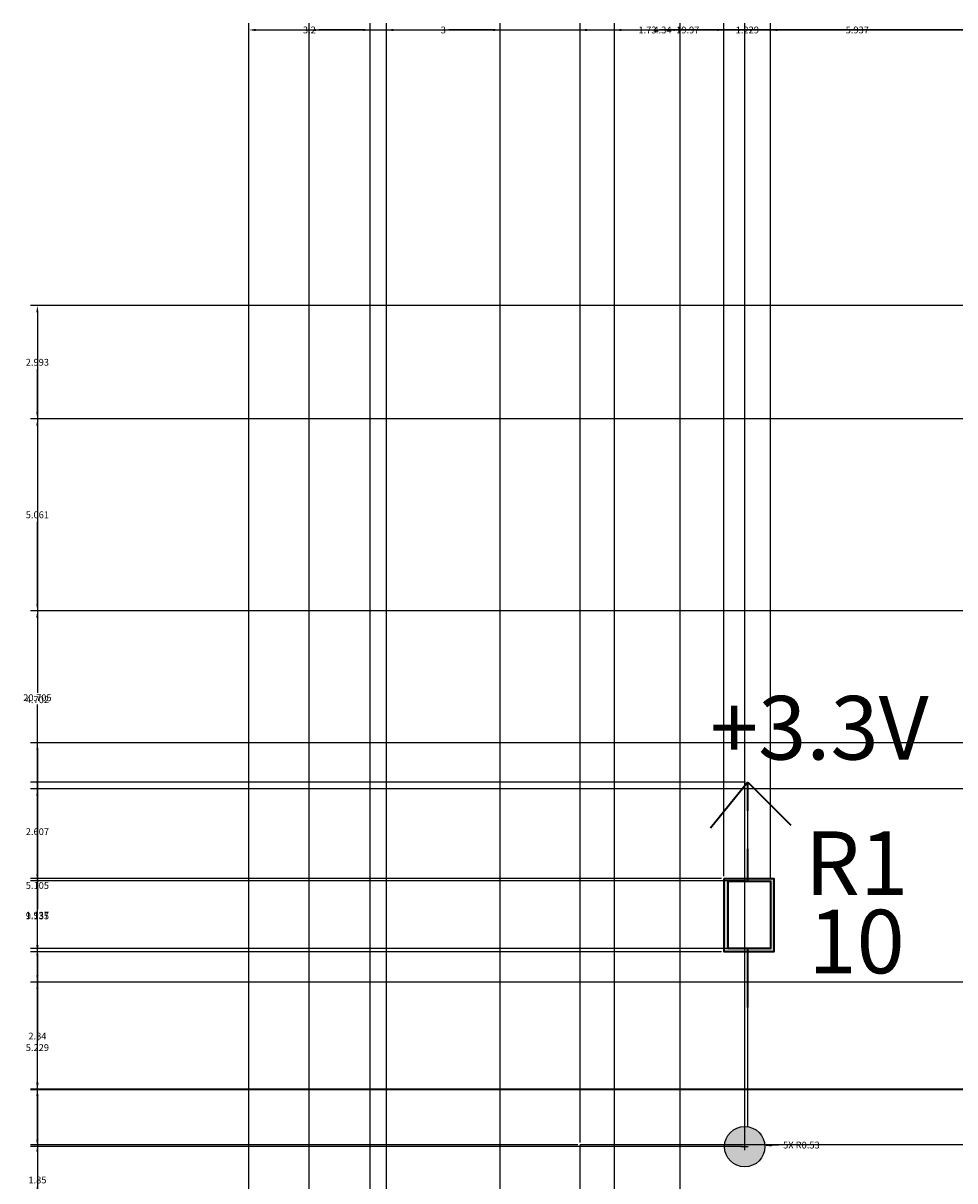
# Model space of a CAD drawing. Units: inches. Extents: x 23 to 132, y 5 to 105.
# Tile 3 of 14: x 23 to 47, y 75 to 105. Entities that reach past the tile are written whole.
import ezdxf

# ---------------------------------------------------------------- set-up
doc = ezdxf.new("R2010")
doc.units = ezdxf.units.IN
doc.header["$MEASUREMENT"] = 0
for name, color, linetype, lineweight in [('A-ANNO-DIMS', 2, 'Continuous', 18), ('E-ANNO-IDEN', 4, 'Continuous', 18), ('E-SYMB', 1, 'Continuous', 35), ('E-SYMB-PATT', 1, 'Continuous', 18), ('E-WIRE', 3, 'Continuous', 25), ('E-WIRE-PATT', 3, 'Continuous', 18)]:
    doc.layers.add(name, color=color, linetype=linetype, lineweight=lineweight)
doc.styles.get("Standard").update_dxf_attribs({"font": 'arial.ttf'})
doc.dimstyles.get("Standard").update_dxf_attribs({"dimtxt": 0.18, "dimasz": 0.18, "dimexe": 0.18, "dimexo": 0.0625, "dimgap": 0.09, "dimtad": 0, "dimtih": 1, "dimtoh": 1, "dimdec": 4, "dimzin": 0, "dimdsep": 46, "dimtxsty": 'Standard', "dimcen": 0.09, "dimadec": 0, "dimazin": 0, "dimtfac": 1, "dimtdec": 4, "dimtofl": 0, "dimtmove": 0, "dimatfit": 3, "dimfxl": 1, "dimtolj": 1, "dimtzin": 0, "dimarcsym": 0})

# ---------------------------------------------------------------- blocks, each defined once
blk = doc.blocks.new('*D2')
at = {"layer": 'A-ANNO-DIMS', "color": 0, "lineweight": -2, "transparency": 16777216}
for p, q in [((28.697, 66.272), (28.697, 105.232)), ((123.211, 99.539), (123.211, 105.232)), ((28.877, 105.052), (75.577, 105.052)), ((123.031, 105.052), (76.33, 105.052))]:
    blk.add_line(p, q, dxfattribs=at)
at = {"layer": 'A-ANNO-DIMS', "color": 0, "transparency": 16777216}
for points in [[(28.877, 105.082), (28.877, 105.022), (28.697, 105.052)], [(123.031, 105.082), (123.031, 105.022), (123.211, 105.052)]]:
    blk.add_solid(points, dxfattribs=at)
at = {"layer": 'Defpoints', "color": 0, "transparency": 16777216}
for p in [(123.211, 105.052), (123.211, 99.477), (28.697, 66.21)]:
    blk.add_point(p, dxfattribs=at)
at = {"layer": 'A-ANNO-DIMS', "color": 0, "transparency": 16777216, "insert": (75.954, 105.052), "char_height": 0.18, "attachment_point": 5}
blk.add_mtext('\\A1;94.51', dxfattribs=at)
blk = doc.blocks.new('*D6')
at = {"layer": 'A-ANNO-DIMS', "color": 0, "lineweight": -2, "transparency": 16777216}
for p, q in [((50.202, 77.095), (22.942, 77.095)), ((23.122, 76.915), (23.122, 47.733)), ((23.122, 18.187), (23.122, 47.369)), ((50.202, 18.007), (22.942, 18.007))]:
    blk.add_line(p, q, dxfattribs=at)
at = {"layer": 'A-ANNO-DIMS', "color": 0, "transparency": 16777216}
for points in [[(23.092, 76.915), (23.152, 76.915), (23.122, 77.095)], [(23.092, 18.187), (23.152, 18.187), (23.122, 18.007)]]:
    blk.add_solid(points, dxfattribs=at)
at = {"layer": 'Defpoints', "color": 0, "transparency": 16777216}
for p in [(23.122, 77.095), (50.265, 77.095), (50.265, 18.007)]:
    blk.add_point(p, dxfattribs=at)
at = {"layer": 'A-ANNO-DIMS', "color": 0, "transparency": 16777216, "insert": (23.122, 47.551), "char_height": 0.18, "attachment_point": 5}
blk.add_mtext('\\A1;59.09', dxfattribs=at)
blk = doc.blocks.new('*D7')
at = {"layer": 'A-ANNO-DIMS', "color": 0, "lineweight": -2, "transparency": 16777216}
for p, q in [((30.295, 73.877), (30.295, 105.232)), ((50.265, 77.157), (50.265, 105.232)), ((30.475, 105.052), (39.895, 105.052)), ((50.085, 105.052), (40.665, 105.052))]:
    blk.add_line(p, q, dxfattribs=at)
at = {"layer": 'A-ANNO-DIMS', "color": 0, "transparency": 16777216}
for points in [[(30.475, 105.082), (30.475, 105.022), (30.295, 105.052)], [(50.085, 105.082), (50.085, 105.022), (50.265, 105.052)]]:
    blk.add_solid(points, dxfattribs=at)
at = {"layer": 'Defpoints', "color": 0, "transparency": 16777216}
for p in [(50.265, 105.052), (50.265, 77.095), (30.295, 73.814)]:
    blk.add_point(p, dxfattribs=at)
at = {"layer": 'A-ANNO-DIMS', "color": 0, "transparency": 16777216, "insert": (40.28, 105.052), "char_height": 0.18, "attachment_point": 5}
blk.add_mtext('\\A1;19.97', dxfattribs=at)
blk = doc.blocks.new('*D12')
at = {"layer": 'A-ANNO-DIMS', "color": 0, "lineweight": -2, "transparency": 16777216}
for p, q in [((64.714, 86.23), (22.942, 86.23)), ((23.122, 86.05), (23.122, 81.845)), ((23.122, 77.275), (23.122, 81.481)), ((64.714, 77.095), (22.942, 77.095))]:
    blk.add_line(p, q, dxfattribs=at)
at = {"layer": 'A-ANNO-DIMS', "color": 0, "transparency": 16777216}
for points in [[(23.092, 86.05), (23.152, 86.05), (23.122, 86.23)], [(23.092, 77.275), (23.152, 77.275), (23.122, 77.095)]]:
    blk.add_solid(points, dxfattribs=at)
at = {"layer": 'Defpoints', "color": 0, "transparency": 16777216}
for p in [(23.122, 86.23), (64.777, 86.23), (64.777, 77.095)]:
    blk.add_point(p, dxfattribs=at)
at = {"layer": 'A-ANNO-DIMS', "color": 0, "transparency": 16777216, "insert": (23.122, 81.663), "char_height": 0.18, "attachment_point": 5}
blk.add_mtext('\\A1;9.135', dxfattribs=at)
blk = doc.blocks.new('*D48')
at = {"layer": 'A-ANNO-DIMS', "color": 0, "lineweight": -2, "transparency": 16777216}
for p, q in [((41.783, 75.637), (41.783, 105.232)), ((47.72, 75.683), (47.72, 105.232)), ((41.963, 105.052), (44.358, 105.052)), ((47.54, 105.052), (45.145, 105.052))]:
    blk.add_line(p, q, dxfattribs=at)
at = {"layer": 'A-ANNO-DIMS', "color": 0, "transparency": 16777216}
for points in [[(41.963, 105.082), (41.963, 105.022), (41.783, 105.052)], [(47.54, 105.082), (47.54, 105.022), (47.72, 105.052)]]:
    blk.add_solid(points, dxfattribs=at)
at = {"layer": 'Defpoints', "color": 0, "transparency": 16777216}
for p in [(47.72, 105.052), (41.783, 75.575), (47.72, 75.621)]:
    blk.add_point(p, dxfattribs=at)
at = {"layer": 'A-ANNO-DIMS', "color": 0, "transparency": 16777216, "insert": (44.752, 105.052), "char_height": 0.18, "attachment_point": 5}
blk.add_mtext('\\A1;5.937', dxfattribs=at)
blk = doc.blocks.new('*D50')
at = {"layer": 'A-ANNO-DIMS', "color": 0, "lineweight": -2, "transparency": 16777216}
for p, q in [((41.236, 82.714), (41.236, 105.232)), ((42.465, 82.649), (42.465, 105.232)), ((41.056, 105.052), (40.876, 105.052)), ((42.645, 105.052), (42.825, 105.052))]:
    blk.add_line(p, q, dxfattribs=at)
at = {"layer": 'A-ANNO-DIMS', "color": 0, "transparency": 16777216}
for points in [[(41.056, 105.082), (41.056, 105.022), (41.236, 105.052)], [(42.645, 105.082), (42.645, 105.022), (42.465, 105.052)]]:
    blk.add_solid(points, dxfattribs=at)
at = {"layer": 'Defpoints', "color": 0, "transparency": 16777216}
for p in [(42.465, 105.052), (41.236, 82.652), (42.465, 82.587)]:
    blk.add_point(p, dxfattribs=at)
at = {"layer": 'A-ANNO-DIMS', "color": 0, "transparency": 16777216, "insert": (41.851, 105.052), "char_height": 0.18, "attachment_point": 5}
blk.add_mtext('\\A1;1.229', dxfattribs=at)
blk = doc.blocks.new('*D51')
at = {"layer": 'A-ANNO-DIMS', "color": 0, "lineweight": -2, "transparency": 16777216}
for p, q in [((41.174, 82.652), (22.942, 82.652)), ((23.122, 82.472), (23.122, 81.865)), ((23.122, 80.895), (23.122, 81.501)), ((41.174, 80.715), (22.942, 80.715))]:
    blk.add_line(p, q, dxfattribs=at)
at = {"layer": 'A-ANNO-DIMS', "color": 0, "transparency": 16777216}
for points in [[(23.092, 82.472), (23.152, 82.472), (23.122, 82.652)], [(23.092, 80.895), (23.152, 80.895), (23.122, 80.715)]]:
    blk.add_solid(points, dxfattribs=at)
at = {"layer": 'Defpoints', "color": 0, "transparency": 16777216}
for p in [(23.122, 82.652), (41.236, 82.652), (41.236, 80.715)]:
    blk.add_point(p, dxfattribs=at)
at = {"layer": 'A-ANNO-DIMS', "color": 0, "transparency": 16777216, "insert": (23.122, 81.683), "char_height": 0.18, "attachment_point": 5}
blk.add_mtext('\\A1;1.937', dxfattribs=at)
blk = doc.blocks.new('*D52')
at = {"layer": 'A-ANNO-DIMS', "color": 0, "lineweight": -2, "transparency": 16777216}
for p, q in [((41.802, 80.803), (22.942, 80.803)), ((23.122, 80.623), (23.122, 78.371)), ((23.122, 75.755), (23.122, 78.007)), ((41.72, 75.575), (22.942, 75.575))]:
    blk.add_line(p, q, dxfattribs=at)
at = {"layer": 'A-ANNO-DIMS', "color": 0, "transparency": 16777216}
for points in [[(23.092, 80.623), (23.152, 80.623), (23.122, 80.803)], [(23.092, 75.755), (23.152, 75.755), (23.122, 75.575)]]:
    blk.add_solid(points, dxfattribs=at)
at = {"layer": 'Defpoints', "color": 0, "transparency": 16777216}
for p in [(23.122, 80.803), (41.865, 80.803), (41.783, 75.575)]:
    blk.add_point(p, dxfattribs=at)
at = {"layer": 'A-ANNO-DIMS', "color": 0, "transparency": 16777216, "insert": (23.122, 78.189), "char_height": 0.18, "attachment_point": 5}
blk.add_mtext('\\A1;5.229', dxfattribs=at)
blk = doc.blocks.new('*D53')
at = {"layer": 'A-ANNO-DIMS', "color": 0, "lineweight": -2, "transparency": 16777216}
for p, q in [((41.802, 85.194), (22.942, 85.194)), ((23.122, 85.014), (23.122, 84.072)), ((23.122, 82.767), (23.122, 83.708)), ((41.802, 82.587), (22.942, 82.587))]:
    blk.add_line(p, q, dxfattribs=at)
at = {"layer": 'A-ANNO-DIMS', "color": 0, "transparency": 16777216}
for points in [[(23.092, 85.014), (23.152, 85.014), (23.122, 85.194)], [(23.092, 82.767), (23.152, 82.767), (23.122, 82.587)]]:
    blk.add_solid(points, dxfattribs=at)
at = {"layer": 'Defpoints', "color": 0, "transparency": 16777216}
for p in [(23.122, 85.194), (41.865, 85.194), (41.865, 82.587)]:
    blk.add_point(p, dxfattribs=at)
at = {"layer": 'A-ANNO-DIMS', "color": 0, "transparency": 16777216, "insert": (23.122, 83.89), "char_height": 0.18, "attachment_point": 5}
blk.add_mtext('\\A1;2.607', dxfattribs=at)
blk = doc.blocks.new('*D54')
at = {"layer": 'A-ANNO-DIMS', "color": 0, "lineweight": -2, "transparency": 16777216}
for p, q in [((37.443, 75.683), (37.443, 105.232)), ((41.783, 75.637), (41.783, 105.232)), ((37.623, 105.052), (39.286, 105.052)), ((41.603, 105.052), (39.94, 105.052))]:
    blk.add_line(p, q, dxfattribs=at)
at = {"layer": 'A-ANNO-DIMS', "color": 0, "transparency": 16777216}
for points in [[(37.623, 105.082), (37.623, 105.022), (37.443, 105.052)], [(41.603, 105.082), (41.603, 105.022), (41.783, 105.052)]]:
    blk.add_solid(points, dxfattribs=at)
at = {"layer": 'Defpoints', "color": 0, "transparency": 16777216}
for p in [(41.783, 105.052), (37.443, 75.621), (41.783, 75.575)]:
    blk.add_point(p, dxfattribs=at)
at = {"layer": 'A-ANNO-DIMS', "color": 0, "transparency": 16777216, "insert": (39.613, 105.052), "char_height": 0.18, "attachment_point": 5}
blk.add_mtext('\\A1;4.34', dxfattribs=at)
blk = doc.blocks.new('*D60')
at = {"layer": 'A-ANNO-DIMS', "color": 0, "lineweight": -2, "transparency": 16777216}
for p, q in [((28.697, 66.272), (28.697, 105.232)), ((31.897, 66.272), (31.897, 105.232)), ((28.877, 105.052), (30.044, 105.052)), ((31.717, 105.052), (30.549, 105.052))]:
    blk.add_line(p, q, dxfattribs=at)
at = {"layer": 'A-ANNO-DIMS', "color": 0, "transparency": 16777216}
for points in [[(28.877, 105.082), (28.877, 105.022), (28.697, 105.052)], [(31.717, 105.082), (31.717, 105.022), (31.897, 105.052)]]:
    blk.add_solid(points, dxfattribs=at)
at = {"layer": 'Defpoints', "color": 0, "transparency": 16777216}
for p in [(31.897, 105.052), (28.697, 66.21), (31.897, 66.21)]:
    blk.add_point(p, dxfattribs=at)
at = {"layer": 'A-ANNO-DIMS', "color": 0, "transparency": 16777216, "insert": (30.297, 105.052), "char_height": 0.18, "attachment_point": 5}
blk.add_mtext('\\A1;3.2', dxfattribs=at)
blk = doc.blocks.new('*D64')
at = {"layer": 'A-ANNO-DIMS', "color": 0, "lineweight": -2, "transparency": 16777216}
for p, q in [((37.381, 75.621), (22.942, 75.621)), ((23.122, 75.441), (23.122, 74.876)), ((23.122, 73.948), (23.122, 74.513)), ((37.3, 73.768), (22.942, 73.768))]:
    blk.add_line(p, q, dxfattribs=at)
at = {"layer": 'A-ANNO-DIMS', "color": 0, "transparency": 16777216}
for points in [[(23.092, 75.441), (23.152, 75.441), (23.122, 75.621)], [(23.092, 73.948), (23.152, 73.948), (23.122, 73.768)]]:
    blk.add_solid(points, dxfattribs=at)
at = {"layer": 'Defpoints', "color": 0, "transparency": 16777216}
for p in [(23.122, 75.621), (37.443, 75.621), (37.363, 73.768)]:
    blk.add_point(p, dxfattribs=at)
at = {"layer": 'A-ANNO-DIMS', "color": 0, "transparency": 16777216, "insert": (23.122, 74.694), "char_height": 0.18, "attachment_point": 5}
blk.add_mtext('\\A1;1.85', dxfattribs=at)
blk = doc.blocks.new('*D67')
at = {"layer": 'A-ANNO-DIMS', "color": 0, "lineweight": -2, "transparency": 16777216}
for p, q in [((38.351, 66.244), (38.351, 105.232)), ((40.084, 66.244), (40.084, 105.232)), ((38.531, 105.052), (38.902, 105.052)), ((39.904, 105.052), (39.533, 105.052))]:
    blk.add_line(p, q, dxfattribs=at)
at = {"layer": 'A-ANNO-DIMS', "color": 0, "transparency": 16777216}
for points in [[(38.531, 105.082), (38.531, 105.022), (38.351, 105.052)], [(39.904, 105.082), (39.904, 105.022), (40.084, 105.052)]]:
    blk.add_solid(points, dxfattribs=at)
at = {"layer": 'Defpoints', "color": 0, "transparency": 16777216}
for p in [(40.084, 105.052), (38.351, 66.181), (40.084, 66.181)]:
    blk.add_point(p, dxfattribs=at)
at = {"layer": 'A-ANNO-DIMS', "color": 0, "transparency": 16777216, "insert": (39.217, 105.052), "char_height": 0.18, "attachment_point": 5}
blk.add_mtext('\\A1;1.73', dxfattribs=at)
blk = doc.blocks.new('*D69')
at = {"layer": 'A-ANNO-DIMS', "color": 0, "lineweight": -2, "transparency": 16777216}
for p, q in [((32.33, 56.687), (32.33, 105.232)), ((35.33, 56.687), (35.33, 105.232)), ((32.51, 105.052), (33.681, 105.052)), ((35.15, 105.052), (33.979, 105.052))]:
    blk.add_line(p, q, dxfattribs=at)
at = {"layer": 'A-ANNO-DIMS', "color": 0, "transparency": 16777216}
for points in [[(32.51, 105.082), (32.51, 105.022), (32.33, 105.052)], [(35.15, 105.082), (35.15, 105.022), (35.33, 105.052)]]:
    blk.add_solid(points, dxfattribs=at)
at = {"layer": 'Defpoints', "color": 0, "transparency": 16777216}
for p in [(35.33, 105.052), (32.33, 56.625), (35.33, 56.625)]:
    blk.add_point(p, dxfattribs=at)
at = {"layer": 'A-ANNO-DIMS', "color": 0, "transparency": 16777216, "insert": (33.83, 105.052), "char_height": 0.18, "attachment_point": 5}
blk.add_mtext('\\A1;3', dxfattribs=at)
blk = doc.blocks.new('*D85')
at = {"layer": 'A-ANNO-DIMS', "color": 0, "lineweight": -2, "transparency": 16777216}
for p, q in [((106.903, 97.776), (22.942, 97.776)), ((23.122, 97.596), (23.122, 87.606)), ((23.122, 77.251), (23.122, 87.242)), ((106.964, 77.071), (22.942, 77.071))]:
    blk.add_line(p, q, dxfattribs=at)
at = {"layer": 'A-ANNO-DIMS', "color": 0, "transparency": 16777216}
for points in [[(23.092, 97.596), (23.152, 97.596), (23.122, 97.776)], [(23.092, 77.251), (23.152, 77.251), (23.122, 77.071)]]:
    blk.add_solid(points, dxfattribs=at)
at = {"layer": 'Defpoints', "color": 0, "transparency": 16777216}
for p in [(23.122, 97.776), (106.965, 97.776), (107.026, 77.071)]:
    blk.add_point(p, dxfattribs=at)
at = {"layer": 'A-ANNO-DIMS', "color": 0, "transparency": 16777216, "insert": (23.122, 87.424), "char_height": 0.18, "attachment_point": 5}
blk.add_mtext('\\A1;20.705', dxfattribs=at)
blk = doc.blocks.new('*D86')
at = {"layer": 'A-ANNO-DIMS', "color": 0, "lineweight": -2, "transparency": 16777216}
for p, q in [((110.027, 79.916), (22.942, 79.916)), ((23.122, 79.736), (23.122, 78.675)), ((23.122, 77.251), (23.122, 78.312)), ((106.964, 77.071), (22.942, 77.071))]:
    blk.add_line(p, q, dxfattribs=at)
at = {"layer": 'A-ANNO-DIMS', "color": 0, "transparency": 16777216}
for points in [[(23.092, 79.736), (23.152, 79.736), (23.122, 79.916)], [(23.092, 77.251), (23.152, 77.251), (23.122, 77.071)]]:
    blk.add_solid(points, dxfattribs=at)
at = {"layer": 'Defpoints', "color": 0, "transparency": 16777216}
for p in [(23.122, 79.916), (110.089, 79.916), (107.026, 77.071)]:
    blk.add_point(p, dxfattribs=at)
at = {"layer": 'A-ANNO-DIMS', "color": 0, "transparency": 16777216, "insert": (23.122, 78.493), "char_height": 0.18, "attachment_point": 5}
blk.add_mtext('\\A1;2.84', dxfattribs=at)
blk = doc.blocks.new('*D87')
at = {"layer": 'A-ANNO-DIMS', "color": 0, "lineweight": -2, "transparency": 16777216}
for p, q in [((110.027, 85.021), (22.942, 85.021)), ((23.122, 84.841), (23.122, 82.65)), ((23.122, 80.096), (23.122, 82.286)), ((110.027, 79.916), (22.942, 79.916))]:
    blk.add_line(p, q, dxfattribs=at)
at = {"layer": 'A-ANNO-DIMS', "color": 0, "transparency": 16777216}
for points in [[(23.092, 84.841), (23.152, 84.841), (23.122, 85.021)], [(23.092, 80.096), (23.152, 80.096), (23.122, 79.916)]]:
    blk.add_solid(points, dxfattribs=at)
at = {"layer": 'Defpoints', "color": 0, "transparency": 16777216}
for p in [(23.122, 85.021), (110.089, 85.021), (110.089, 79.916)]:
    blk.add_point(p, dxfattribs=at)
at = {"layer": 'A-ANNO-DIMS', "color": 0, "transparency": 16777216, "insert": (23.122, 82.468), "char_height": 0.18, "attachment_point": 5}
blk.add_mtext('\\A1;5.105', dxfattribs=at)
blk = doc.blocks.new('*D88')
at = {"layer": 'A-ANNO-DIMS', "color": 0, "lineweight": -2, "transparency": 16777216}
for p, q in [((110.027, 89.722), (22.942, 89.722)), ((23.122, 89.542), (23.122, 87.554)), ((23.122, 85.201), (23.122, 87.19)), ((110.027, 85.021), (22.942, 85.021))]:
    blk.add_line(p, q, dxfattribs=at)
at = {"layer": 'A-ANNO-DIMS', "color": 0, "transparency": 16777216}
for points in [[(23.092, 89.542), (23.152, 89.542), (23.122, 89.722)], [(23.092, 85.201), (23.152, 85.201), (23.122, 85.021)]]:
    blk.add_solid(points, dxfattribs=at)
at = {"layer": 'Defpoints', "color": 0, "transparency": 16777216}
for p in [(23.122, 89.722), (110.089, 89.722), (110.089, 85.021)]:
    blk.add_point(p, dxfattribs=at)
at = {"layer": 'A-ANNO-DIMS', "color": 0, "transparency": 16777216, "insert": (23.122, 87.372), "char_height": 0.18, "attachment_point": 5}
blk.add_mtext('\\A1;4.702', dxfattribs=at)
blk = doc.blocks.new('*D89')
at = {"layer": 'A-ANNO-DIMS', "color": 0, "lineweight": -2, "transparency": 16777216}
for p, q in [((110.298, 94.783), (22.942, 94.783)), ((23.122, 94.603), (23.122, 92.435)), ((23.122, 89.902), (23.122, 92.071)), ((110.027, 89.722), (22.942, 89.722))]:
    blk.add_line(p, q, dxfattribs=at)
at = {"layer": 'A-ANNO-DIMS', "color": 0, "transparency": 16777216}
for points in [[(23.092, 94.603), (23.152, 94.603), (23.122, 94.783)], [(23.092, 89.902), (23.152, 89.902), (23.122, 89.722)]]:
    blk.add_solid(points, dxfattribs=at)
at = {"layer": 'Defpoints', "color": 0, "transparency": 16777216}
for p in [(23.122, 94.783), (110.36, 94.783), (110.089, 89.722)]:
    blk.add_point(p, dxfattribs=at)
at = {"layer": 'A-ANNO-DIMS', "color": 0, "transparency": 16777216, "insert": (23.122, 92.253), "char_height": 0.18, "attachment_point": 5}
blk.add_mtext('\\A1;5.061', dxfattribs=at)
blk = doc.blocks.new('*D90')
at = {"layer": 'A-ANNO-DIMS', "color": 0, "lineweight": -2, "transparency": 16777216}
for p, q in [((106.903, 97.776), (22.942, 97.776)), ((23.122, 97.596), (23.122, 96.462)), ((23.122, 94.963), (23.122, 96.098)), ((110.298, 94.783), (22.942, 94.783))]:
    blk.add_line(p, q, dxfattribs=at)
at = {"layer": 'A-ANNO-DIMS', "color": 0, "transparency": 16777216}
for points in [[(23.092, 97.596), (23.152, 97.596), (23.122, 97.776)], [(23.092, 94.963), (23.152, 94.963), (23.122, 94.783)]]:
    blk.add_solid(points, dxfattribs=at)
at = {"layer": 'Defpoints', "color": 0, "transparency": 16777216}
for p in [(23.122, 97.776), (106.965, 97.776), (110.36, 94.783)]:
    blk.add_point(p, dxfattribs=at)
at = {"layer": 'A-ANNO-DIMS', "color": 0, "transparency": 16777216, "insert": (23.122, 96.28), "char_height": 0.18, "attachment_point": 5}
blk.add_mtext('\\A1;2.993', dxfattribs=at)
blk = doc.blocks.new('*D97')
at = {"layer": 'A-ANNO-DIMS', "color": 0, "lineweight": -2, "transparency": 16777216}
for p, q in [((41.693, 75.575), (41.873, 75.575)), ((41.783, 75.485), (41.783, 75.665)), ((42.675, 75.616), (42.495, 75.608))]:
    blk.add_line(p, q, dxfattribs=at)
at = {"layer": 'A-ANNO-DIMS', "color": 0, "transparency": 16777216}
blk.add_solid([(42.493, 75.638), (42.496, 75.578), (42.315, 75.599)], dxfattribs=at)
at = {"layer": 'Defpoints', "color": 0, "transparency": 16777216}
for p in [(41.783, 75.575), (42.315, 75.599)]:
    blk.add_point(p, dxfattribs=at)
at = {"layer": 'A-ANNO-DIMS', "color": 0, "transparency": 16777216, "insert": (43.278, 75.616), "char_height": 0.18, "attachment_point": 5}
blk.add_mtext('\\A1;5X R0.53', dxfattribs=at)

msp = doc.modelspace()

# ---------------------------------------------------------------- hatches: boundary and pattern name
at = {"layer": 'E-SYMB-PATT'}
h = msp.add_hatch(color=256, dxfattribs=at)
h.dxf.hatch_style = 1
h.paths.add_polyline_path([(42.5487, 82.652), (41.2363, 82.652), (41.2363, 80.7149), (42.5487, 80.7149)])
h.paths.add_polyline_path([(41.3492, 80.8053), (41.3492, 82.5866), (42.4654, 82.5866), (42.4654, 80.8053)], flags=16)
at = {"layer": 'E-WIRE-PATT'}
h = msp.add_hatch(color=256, dxfattribs=at)
h.dxf.hatch_style = 1
h.paths.add_polyline_path([(41.2522, 75.6207), (42.3136, 75.6207, 0.9167819)])
h.paths.add_polyline_path([(42.3156, 75.5745, 0.0216975), (42.3136, 75.6207), (41.2522, 75.6207, 0.0216975), (41.2502, 75.5745, 1)])
h.paths.add_polyline_path([(37.4432, 74.2949), (37.4432, 73.8144), (37.4432, 73.2415, 0.3706245), (37.8957, 73.7682, 0.3706245)])
h.paths.add_polyline_path([(37.4432, 74.2949, 0.4331755), (36.8323, 73.8144), (37.4432, 73.8144)])
h.paths.add_polyline_path([(37.4432, 73.8144), (36.8323, 73.8144, 0.0216975), (36.8302, 73.7682, 0.4591888), (37.4432, 73.2415)])

# ---------------------------------------------------------------- linework, layer by layer
at = {"layer": 'E-SYMB'}
for p, q in [((41.8647, 85.1937), (40.8827, 83.9847)), ((41.8647, 84.4384), (41.8647, 85.1937)), ((41.8647, 85.1937), (43.0034, 84.0647)), ((41.8647, 82.5866), (41.8647, 83.4378)), ((41.8647, 80.8031), (41.8647, 80.8053)), ((41.8647, 79.2453), (41.8647, 80.8031))]:
    msp.add_line(p, q, dxfattribs=at)
for points in [[(41.2363, 82.652), (42.5487, 82.652), (42.5487, 80.7149), (41.2363, 80.7149)], [(41.3492, 82.5866), (42.4654, 82.5866), (42.4654, 80.8053), (41.3492, 80.8053)]]:
    msp.add_lwpolyline(points, close=True, dxfattribs=at)
at = {"layer": 'E-WIRE'}
for p, q in [((41.8647, 83.4378), (41.8647, 84.4384)), ((41.8647, 76.101), (41.8647, 79.2453)), ((37.4432, 73.8144), (37.4432, 75.6207)), ((47.7202, 75.6207), (37.4432, 75.6207))]:
    msp.add_line(p, q, dxfattribs=at)
msp.add_circle((41.7829, 75.5745), 0.5327, dxfattribs=at)

# ---------------------------------------------------------------- texts
at = {"layer": 'E-ANNO-IDEN'}
for s, p in [('+3.3V', (40.8644, 85.792)), ('R1', (43.3689, 82.2182)), ('10', (43.461, 80.1489))]:
    msp.add_text(s, height=1.67943, dxfattribs=at).set_placement(p)

# ---------------------------------------------------------------- dimensions: what is measured, and where the dimension line sits
at = {"layer": 'A-ANNO-DIMS'}
for base, p1, p2, override, picture, middle in [((123.2107, 105.052), (28.6965, 66.2099), (123.2107, 99.477), {"dimdec": 2, "dimlfac": 1, "dimrnd": 0, "dimzin": 0, "dimdsep": 46, "dimlunit": 2}, '*D2', (75.9536, 105.052)), ((31.8965, 105.052), (28.6965, 66.2099), (31.8965, 66.2099), {"dimdec": 1, "dimlfac": 1, "dimrnd": 0, "dimzin": 0, "dimdsep": 46, "dimlunit": 2}, '*D60', (30.2965, 105.052)), ((50.2646, 105.052), (30.2954, 73.8144), (50.2646, 77.095), {"dimdec": 2, "dimlfac": 1, "dimrnd": 0, "dimzin": 0, "dimdsep": 46, "dimlunit": 2}, '*D7', (40.28, 105.052)), ((35.3299, 105.052), (32.3299, 56.6249), (35.3299, 56.6249), {"dimdec": 0, "dimlfac": 1, "dimrnd": 0, "dimzin": 0, "dimdsep": 46, "dimlunit": 2}, '*D69', (33.8299, 105.052)), ((41.7829, 105.052), (37.4432, 75.6207), (41.7829, 75.5745), {"dimdec": 2, "dimlfac": 1, "dimrnd": 0, "dimzin": 0, "dimdsep": 46, "dimlunit": 2}, '*D54', (39.613, 105.052)), ((40.0835, 105.052), (38.3512, 66.1814), (40.0835, 66.1814), {"dimdec": 2, "dimlfac": 1, "dimrnd": 0, "dimzin": 0, "dimdsep": 46, "dimlunit": 2}, '*D67', (39.2174, 105.052)), ((42.4654, 105.052), (41.2363, 82.652), (42.4654, 82.5866), {"dimdec": 3, "dimlfac": 1, "dimrnd": 0, "dimzin": 0, "dimdsep": 46, "dimlunit": 2}, '*D50', (41.8508, 105.052)), ((47.7202, 105.052), (41.7829, 75.5745), (47.7202, 75.6207), {"dimdec": 3, "dimlfac": 1, "dimrnd": 0, "dimzin": 0, "dimdsep": 46, "dimlunit": 2}, '*D48', (44.7515, 105.052))]:
    dim = msp.add_linear_dim(base=base, p1=p1, p2=p2, dimstyle='Standard', override=override, dxfattribs=at)
    dim.commit()
    dim.dimension.update_dxf_attribs({"geometry": picture, "text_midpoint": middle})
for base, p1, p2, override, picture, middle in [((23.1215, 97.7764), (107.026, 77.0711), (106.9652, 97.7764), {"dimdec": 3, "dimlfac": 1, "dimrnd": 0, "dimzin": 0, "dimdsep": 46, "dimlunit": 2}, '*D85', (23.1215, 87.4238)), ((23.1215, 97.7764), (110.36, 94.7833), (106.9652, 97.7764), {"dimdec": 3, "dimlfac": 1, "dimrnd": 0, "dimzin": 0, "dimdsep": 46, "dimlunit": 2}, '*D90', (23.1215, 96.2798)), ((23.1215, 94.7833), (110.0892, 89.7224), (110.36, 94.7833), {"dimdec": 3, "dimlfac": 1, "dimrnd": 0, "dimzin": 0, "dimdsep": 46, "dimlunit": 2}, '*D89', (23.1215, 92.2528)), ((23.12152, 89.7224), (110.08916, 85.02085), (110.08916, 89.7224), {"dimdec": 3, "dimlfac": 1, "dimrnd": 0, "dimzin": 0, "dimdsep": 46, "dimlunit": 2}, '*D88', (23.12152, 87.37162)), ((23.1215, 86.2302), (64.7769, 77.095), (64.7769, 86.2302), {"dimdec": 3, "dimlfac": 1, "dimrnd": 0, "dimzin": 0, "dimdsep": 46, "dimlunit": 2}, '*D12', (23.1215, 81.6626)), ((23.1215, 85.1937), (41.8647, 82.5866), (41.8647, 85.1937), {"dimdec": 3, "dimlfac": 1, "dimrnd": 0, "dimzin": 0, "dimdsep": 46, "dimlunit": 2}, '*D53', (23.1215, 83.8902)), ((23.1215, 85.0209), (110.0892, 79.9158), (110.0892, 85.0209), {"dimdec": 3, "dimlfac": 1, "dimrnd": 0, "dimzin": 0, "dimdsep": 46, "dimlunit": 2}, '*D87', (23.1215, 82.4683)), ((23.1215, 82.652), (41.2363, 80.7149), (41.2363, 82.652), {"dimdec": 3, "dimlfac": 1, "dimrnd": 0, "dimzin": 0, "dimdsep": 46, "dimlunit": 2}, '*D51', (23.1215, 81.6835)), ((23.1215, 80.8031), (41.7829, 75.5745), (41.8647, 80.8031), {"dimdec": 3, "dimlfac": 1, "dimrnd": 0, "dimzin": 0, "dimdsep": 46, "dimlunit": 2}, '*D52', (23.1215, 78.1888)), ((23.1215, 79.9158), (107.026, 77.0711), (110.0892, 79.9158), {"dimdec": 2, "dimlfac": 1, "dimrnd": 0, "dimzin": 0, "dimdsep": 46, "dimlunit": 2}, '*D86', (23.1215, 78.4935)), ((23.1215, 77.095), (50.2646, 18.0066), (50.2646, 77.095), {"dimdec": 2, "dimlfac": 1, "dimrnd": 0, "dimzin": 0, "dimdsep": 46, "dimlunit": 2}, '*D6', (23.1215, 47.5508)), ((23.1215, 75.6207), (37.363, 73.7682), (37.4432, 75.6207), {"dimdec": 2, "dimlfac": 1, "dimrnd": 0, "dimzin": 0, "dimdsep": 46, "dimlunit": 2}, '*D64', (23.1215, 74.6945))]:
    dim = msp.add_linear_dim(base=base, p1=p1, p2=p2, angle=90, dimstyle='Standard', override=override, dxfattribs=at)
    dim.commit()
    dim.dimension.update_dxf_attribs({"geometry": picture, "text_midpoint": middle})
dim = msp.add_radius_dim(center=(41.7829, 75.5745), mpoint=(42.315, 75.5993), text='5X <>', dimstyle='Standard', override={"dimdec": 2, "dimlfac": 1, "dimrnd": 0, "dimzin": 0, "dimdsep": 46, "dimlunit": 2}, dxfattribs=at)
dim.commit()
dim.dimension.update_dxf_attribs({"geometry": '*D97', "text_midpoint": (43.278, 75.616)})

doc.saveas('drawing.dxf')
